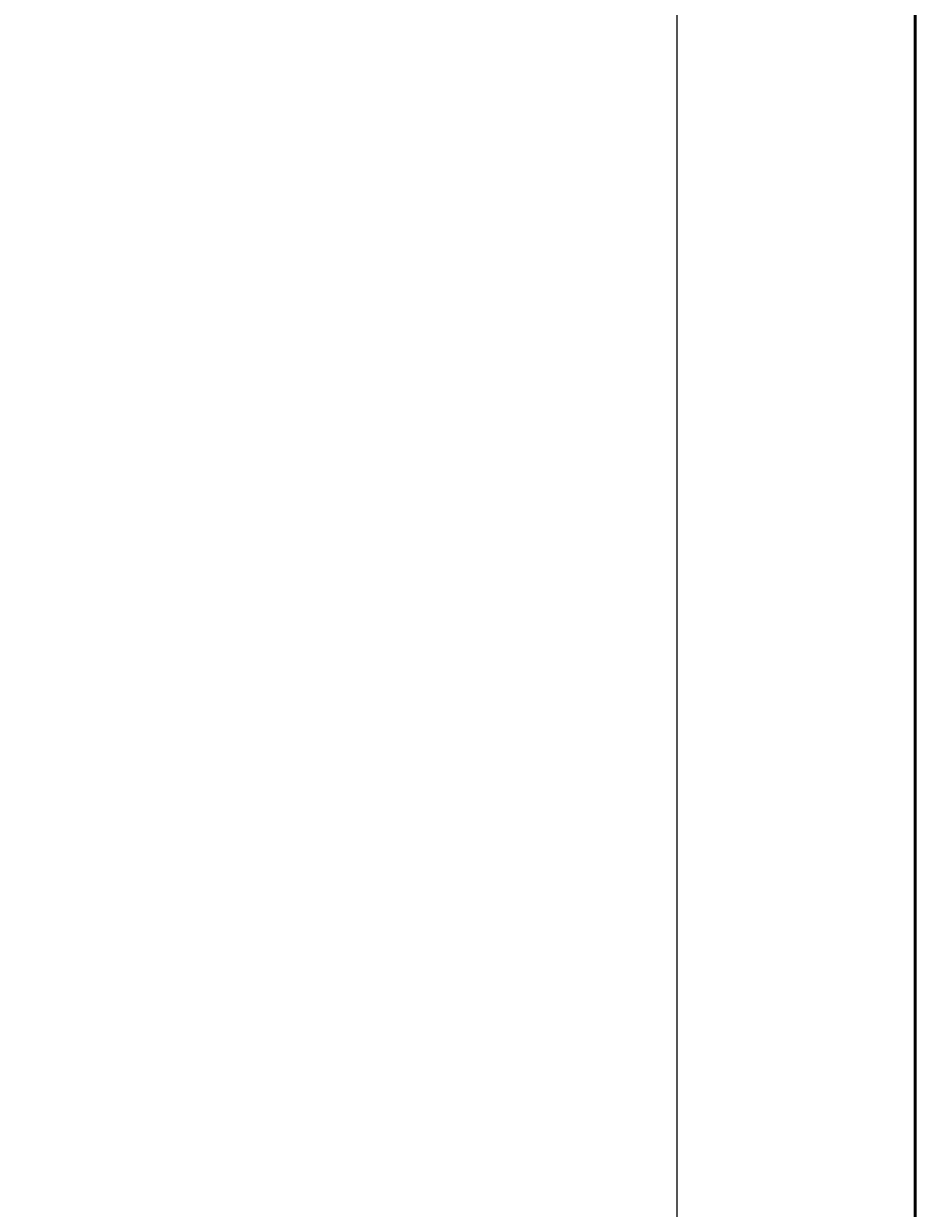
# Model space of a CAD drawing. Units: inches. Extents: x 0 to 281, y -535 to 46.
# Tile 18 of 22: x 134 to 156, y -66 to -36. Entities that reach past the tile are written whole.
import ezdxf

# ---------------------------------------------------------------- set-up
doc = ezdxf.new("R2010")
doc.units = ezdxf.units.IN
doc.header["$MEASUREMENT"] = 0
doc.layers.add('A-ANNO-DIMS', color=2, linetype='Continuous', lineweight=18)
doc.layers.add('A-WALL', color=7, linetype='Continuous', lineweight=50)
doc.styles.get("Standard").update_dxf_attribs({"font": 'arial.ttf'})
doc.dimstyles.get("Standard").update_dxf_attribs({"dimtxt": 0.18, "dimasz": 0.18, "dimexe": 0.18, "dimexo": 0.0625, "dimgap": 0.09, "dimtad": 0, "dimtih": 1, "dimtoh": 1, "dimdec": 0, "dimzin": 0, "dimdsep": 46, "dimlunit": 3, "dimtxsty": 'Standard', "dimcen": 0.09, "dimadec": 0, "dimazin": 0, "dimtfac": 1, "dimtdec": 0, "dimtofl": 0, "dimtmove": 0, "dimatfit": 3, "dimfxl": 1, "dimtolj": 1, "dimtzin": 0, "dimarcsym": 0})

# ---------------------------------------------------------------- blocks, each defined once
blk = doc.blocks.new('*D45')
at = {"layer": 'A-ANNO-DIMS', "color": 0, "lineweight": -2, "transparency": 16777216}
for p, q in [((114.459, -263.348), (114.459, 46.219)), ((114.639, 46.039), (132.13, 46.039)), ((150.279, 46.039), (132.788, 46.039)), ((150.459, -263.348), (150.459, 46.219))]:
    blk.add_line(p, q, dxfattribs=at)
at = {"layer": 'A-ANNO-DIMS', "color": 0, "transparency": 16777216}
for points in [[(114.639, 46.069), (114.639, 46.009), (114.459, 46.039)], [(150.279, 46.069), (150.279, 46.009), (150.459, 46.039)]]:
    blk.add_solid(points, dxfattribs=at)
at = {"layer": 'Defpoints', "color": 0, "transparency": 16777216}
for p in [(150.459, 46.039), (114.459, -263.411), (150.459, -263.411)]:
    blk.add_point(p, dxfattribs=at)
at = {"layer": 'A-ANNO-DIMS', "color": 0, "transparency": 16777216, "insert": (132.459, 46.039), "char_height": 0.18, "attachment_point": 5}
blk.add_mtext('\\A1;3\'-0"', dxfattribs=at)
blk = doc.blocks.new('*D47')
at = {"layer": 'A-ANNO-DIMS', "color": 0, "lineweight": -2, "transparency": 16777216}
for p, q in [((114.459, -392.348), (114.459, 46.219)), ((114.639, 46.039), (132.13, 46.039)), ((150.279, 46.039), (132.788, 46.039)), ((150.459, -392.348), (150.459, 46.219))]:
    blk.add_line(p, q, dxfattribs=at)
at = {"layer": 'A-ANNO-DIMS', "color": 0, "transparency": 16777216}
for points in [[(114.639, 46.069), (114.639, 46.009), (114.459, 46.039)], [(150.279, 46.069), (150.279, 46.009), (150.459, 46.039)]]:
    blk.add_solid(points, dxfattribs=at)
at = {"layer": 'Defpoints', "color": 0, "transparency": 16777216}
for p in [(150.459, 46.039), (114.459, -392.411), (150.459, -392.411)]:
    blk.add_point(p, dxfattribs=at)
at = {"layer": 'A-ANNO-DIMS', "color": 0, "transparency": 16777216, "insert": (132.459, 46.039), "char_height": 0.18, "attachment_point": 5}
blk.add_mtext('\\A1;3\'-0"', dxfattribs=at)

msp = doc.modelspace()

# ---------------------------------------------------------------- linework, layer by layer
at = {"layer": 'A-WALL'}
msp.add_line((156.459, 18.589), (156.459, -131.411), dxfattribs=at)

# ---------------------------------------------------------------- dimensions: what is measured, and where the dimension line sits
at = {"layer": 'A-ANNO-DIMS'}
for p1, p2, picture in [((114.459, -263.411), (150.459, -263.411), '*D45'), ((114.459, -392.411), (150.459, -392.411), '*D47')]:
    dim = msp.add_linear_dim(base=(150.459, 46.039), p1=p1, p2=p2, dimstyle='Standard', override={"dimdec": 1, "dimlfac": 1, "dimrnd": 0, "dimzin": 1, "dimdsep": 46, "dimlunit": 4, "dimfrac": 2}, dxfattribs=at)
    dim.commit()
    dim.dimension.update_dxf_attribs({"geometry": picture, "text_midpoint": (132.459, 46.039)})

doc.saveas('drawing.dxf')
